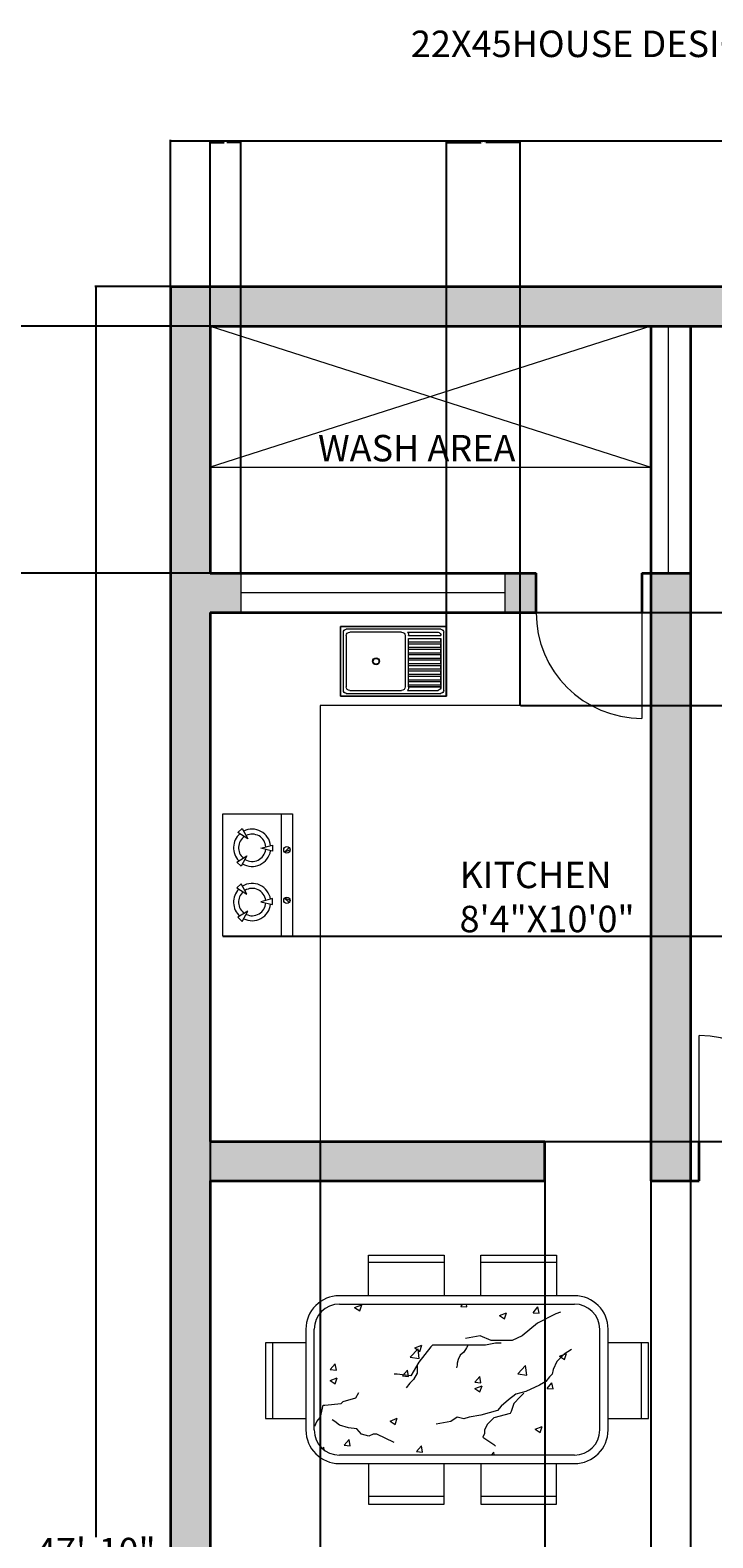
# Model space of a CAD drawing. Units: inches. Extents: x 37 to 706, y -568 to 110.
# Tile 22 of 24: x 362 to 517, y -233 to 110. Entities that reach past the tile are written whole.
import ezdxf

# ---------------------------------------------------------------- set-up
doc = ezdxf.new("R2010")
doc.units = ezdxf.units.IN
doc.header["$MEASUREMENT"] = 0
for name, color, linetype, lineweight in [('A-ANNO-DIMS', 2, 'Continuous', 18), ('A-ANNO-TEXT', 7, 'Continuous', 18), ('A-AREA-IDEN', 7, 'Continuous', 18), ('A-DOOR', 4, 'Continuous', 18), ('A-EQPM', 8, 'Continuous', 18), ('A-FLOR-CASE', 9, 'Continuous', 18), ('A-FLOR-FIXT', 9, 'Continuous', 18), ('A-FLOR-OPEN', 8, 'Continuous', 13), ('A-FURN', 8, 'Continuous', 13), ('A-GLAZ', 4, 'Continuous', 18), ('A-WALL', 7, 'Continuous', 35), ('A-WALL-PATT', 252, 'Continuous', 13)]:
    doc.layers.add(name, color=color, linetype=linetype, lineweight=lineweight)
doc.styles.get("Standard").update_dxf_attribs({"font": 'arial.ttf'})
doc.dimstyles.get("Standard").update_dxf_attribs({"dimtxt": 0.18, "dimasz": 0.18, "dimexe": 0.18, "dimexo": 0.0625, "dimgap": 0.09, "dimtad": 0, "dimtih": 1, "dimtoh": 1, "dimdec": 0, "dimzin": 0, "dimdsep": 46, "dimlunit": 3, "dimtxsty": 'Standard', "dimcen": 0.09, "dimadec": 0, "dimazin": 0, "dimtfac": 1, "dimtdec": 0, "dimtofl": 0, "dimtmove": 0, "dimatfit": 3, "dimfxl": 1, "dimtolj": 1, "dimtzin": 0, "dimarcsym": 0})

# ---------------------------------------------------------------- blocks, each defined once
blk = doc.blocks.new('М12 540х820')
for p, q in [((0, 540), (-820, 540)), ((-820, 540), (-820, 0)), ((-798, 495), (-798, 45)), ((-45, 517), (-775, 517)), ((-775, 468), (-775, 72)), ((-348, 495), (-748, 495)), ((-320, 468), (-320, 72)), ((-302, 495), (-65, 495)), ((-294, 468), (-294, 472)), ((-294, 468), (-45, 468)), ((-45, 470), (-45, 468)), ((-22, 45), (-22, 495)), ((0, 0), (0, 540)), ((-294, 447), (-45, 447)), ((-294, 420), (-294, 447)), ((-294, 420), (-45, 420)), ((-294, 405), (-45, 405)), ((-294, 378), (-294, 405)), ((-294, 378), (-45, 378)), ((-294, 336), (-294, 363)), ((-294, 363), (-45, 363)), ((-45, 420), (-45, 447)), ((-45, 378), (-45, 405)), ((-45, 336), (-45, 363)), ((-294, 336), (-45, 336)), ((-294, 295), (-294, 322)), ((-294, 322), (-45, 322)), ((-294, 295), (-45, 295)), ((-294, 253), (-294, 280)), ((-294, 280), (-45, 280)), ((-294, 253), (-45, 253)), ((-294, 211), (-294, 238)), ((-294, 238), (-45, 238)), ((-45, 295), (-45, 322)), ((-45, 253), (-45, 280)), ((-45, 211), (-45, 238)), ((-294, 211), (-45, 211)), ((-294, 170), (-294, 197)), ((-294, 197), (-45, 197)), ((-294, 170), (-45, 170)), ((-294, 128), (-294, 155)), ((-294, 155), (-45, 155)), ((-294, 128), (-45, 128)), ((-45, 170), (-45, 197)), ((-45, 128), (-45, 155)), ((-820, 0), (0, 0)), ((-775, 22), (-45, 22)), ((-748, 45), (-348, 45)), ((-302, 45), (-65, 45)), ((-294, 114), (-45, 114)), ((-294, 87), (-294, 114)), ((-294, 87), (-45, 87)), ((-294, 72), (-45, 72)), ((-45, 87), (-45, 114)), ((-45, 70), (-45, 72))]:
    blk.add_line(p, q)
at = {"ltscale": 0.06}
for p, q in [((-820, 0), (-820, 540)), ((-820, 540), (0, 540)), ((0, 540), (0, 537)), ((0, 537), (0, 0)), ((-294, 447), (-45, 447)), ((-294, 405), (-294, 447)), ((-294, 363), (-294, 405)), ((-294, 322), (-294, 363)), ((-45, 447), (-45, 420)), ((-45, 420), (-45, 378)), ((-45, 378), (-45, 336)), ((-294, 280), (-294, 322)), ((-294, 238), (-294, 280)), ((-294, 197), (-294, 238)), ((-45, 336), (-45, 295)), ((-45, 295), (-45, 253)), ((-45, 253), (-45, 211)), ((-294, 155), (-294, 197)), ((-294, 114), (-294, 155)), ((-45, 211), (-45, 170)), ((-45, 170), (-45, 128)), ((-45, 128), (-45, 87)), ((0, 0), (-820, 0)), ((-294, 72), (-294, 114)), ((-45, 72), (-294, 72)), ((-45, 87), (-45, 72))]:
    blk.add_line(p, q, dxfattribs=at)
at = {"extrusion": (0, 0, -1)}
for centre, major_axis, start_param, end_param in [((-775, 495), (-15.9, 15.9), -0.785398, 0.785398), ((-775, 495), (-15.9, 15.9), -0.785398, 0.785398), ((-748, 468), (-19.1, -19.1), 0.785398, 2.356194), ((-748, 468), (-19.1, -19.1), 0.785398, 2.356194), ((-348, 468), (-19.1, 19.1), 0.785398, 2.356194), ((-348, 468), (-19.1, 19.1), 0.785398, 2.356194), ((-343, 468), (-35, 35), 1.779263, 2.356194), ((-343, 468), (-35, 35), 1.779263, 2.356192), ((-343, 468), (-35, 35), 2.356192, 2.356194), ((-72, 469), (-19.3, 19.3), 1.0328, 2.38382), ((-72, 469), (-19.3, 19.3), 1.0328, 1.064673), ((-72, 469), (-19.3, 19.3), 1.064673, 2.328569), ((-45, 495), (-15.9, -15.9), 2.356194, 3.926991), ((-45, 495), (-15.9, -15.9), 2.356194, 3.926991), ((-72, 469), (-19.3, 19.3), 2.328569, 2.38382), ((-545, 270), (-19.1, -19.1), 3.926991, 10.210176), ((-545, 270), (-19.1, -19.1), 3.926991, 10.210176), ((-545, 270), (-15.9, -15.9), 3.926991, 10.210176), ((-545, 270), (-15.9, -15.9), 3.926991, 10.210176), ((-775, 45), (-15.9, -15.9), 5.497787, 7.068583), ((-775, 45), (-15.9, -15.9), 5.497787, 7.068583), ((-748, 72), (-19.1, 19.1), 3.926991, 5.497787), ((-748, 72), (-19.1, 19.1), 3.926991, 5.497787), ((-348, 72), (-19.1, -19.1), 3.926991, 5.497787), ((-348, 72), (-19.1, -19.1), 3.926991, 5.497787), ((-343, 72), (-35, -35), 3.926991, 4.503922), ((-343, 72), (-35, -35), 3.926991, 4.503922), ((-72, 71), (-19.3, -19.3), 3.899365, 5.250385), ((-72, 71), (-19.3, -19.3), 5.218512, 5.250385), ((-72, 71), (-19.3, -19.3), 3.954617, 5.218512), ((-72, 71), (-19.3, -19.3), 3.899365, 3.954617), ((-45, 45), (-15.9, 15.9), 2.356194, 3.926991), ((-45, 45), (-15.9, 15.9), 2.356194, 3.926991)]:
    blk.add_ellipse(centre, major_axis=major_axis, ratio=1, start_param=start_param, end_param=end_param, dxfattribs=at)
blk = doc.blocks.new('*D4')
at = {"layer": 'A-ANNO-DIMS', "color": 0, "lineweight": -2, "transparency": 16777216}
for p, q in [((393.96, 51.35), (393.96, 84.59)), ((394.14, 84.41), (523.01, 84.41)), ((672.78, 84.41), (543.91, 84.41)), ((672.96, 51.35), (672.96, 84.59))]:
    blk.add_line(p, q, dxfattribs=at)
at = {"layer": 'A-ANNO-DIMS', "color": 0, "transparency": 16777216}
for points in [[(394.14, 84.44), (394.14, 84.38), (393.96, 84.41)], [(672.78, 84.44), (672.78, 84.38), (672.96, 84.41)]]:
    blk.add_solid(points, dxfattribs=at)
at = {"layer": 'Defpoints', "color": 0, "transparency": 16777216}
for p in [(672.96, 84.41), (393.96, 51.29), (672.96, 51.29)]:
    blk.add_point(p, dxfattribs=at)
at = {"layer": 'A-ANNO-DIMS', "color": 0, "transparency": 16777216, "insert": (533.46, 84.41), "char_height": 6, "attachment_point": 5}
blk.add_mtext('\\A1;23\'-3"', dxfattribs=at)
blk = doc.blocks.new('*D5')
at = {"layer": 'A-ANNO-DIMS', "color": 0, "lineweight": -2, "transparency": 16777216}
for p, q in [((393.9, 51.29), (376.84, 51.29)), ((377.02, 51.11), (377.02, -232.56)), ((377.02, -522.53), (377.02, -238.86)), ((393.9, -522.71), (376.84, -522.71))]:
    blk.add_line(p, q, dxfattribs=at)
at = {"layer": 'A-ANNO-DIMS', "color": 0, "transparency": 16777216}
for points in [[(376.99, 51.11), (377.05, 51.11), (377.02, 51.29)], [(376.99, -522.53), (377.05, -522.53), (377.02, -522.71)]]:
    blk.add_solid(points, dxfattribs=at)
at = {"layer": 'Defpoints', "color": 0, "transparency": 16777216}
for p in [(393.96, 51.29), (377.02, -522.71), (393.96, -522.71)]:
    blk.add_point(p, dxfattribs=at)
at = {"layer": 'A-ANNO-DIMS', "color": 0, "transparency": 16777216, "insert": (377.02, -235.71), "char_height": 6, "attachment_point": 5}
blk.add_mtext('\\A1;47\'-10"', dxfattribs=at)
blk = doc.blocks.new('DINING-SET-6')
for p, q in [((23.4, 47.29), (23.4, 56.48)), ((23.4, 56.48), (40.55, 56.48)), ((40.55, 54.8), (23.4, 54.8)), ((40.55, 56.48), (40.55, 47.29)), ((48.93, 47.29), (48.93, 56.48)), ((48.93, 56.48), (66.08, 56.48)), ((66.08, 54.8), (48.93, 54.8)), ((66.08, 56.48), (66.08, 47.29)), ((70.16, 47.29), (16.81, 47.29)), ((16.81, 45.39), (70.16, 45.39)), ((20.27, 44.63), (21.87, 45.24)), ((20.27, 44.63), (21.41, 43.86)), ((21.41, 43.86), (21.87, 45.24)), ((44.37, 44.86), (44.81, 45.39)), ((44.37, 44.86), (45.74, 44.74)), ((45.74, 44.74), (45.62, 45.39)), ((60.77, 43.43), (61.87, 44.74)), ((62.14, 43.31), (61.87, 44.74)), ((53.13, 42.8), (54.73, 43.41)), ((53.13, 42.8), (54.27, 42.03)), ((54.27, 42.03), (54.73, 43.41)), ((60.77, 43.43), (62.14, 43.31)), ((65.93, 43.13), (61.79, 41.06)), ((66.97, 43.54), (65.93, 43.13)), ((9.18, 39.67), (9.18, 16.81)), ((11.09, 16.81), (11.09, 39.67)), ((46.25, 37.75), (45.42, 37.54)), ((48.74, 38.16), (46.25, 37.75)), ((51.22, 37.13), (48.74, 38.16)), ((58.27, 38.16), (55.99, 37.13)), ((61.79, 41.06), (58.27, 38.16)), ((75.87, 39.67), (75.87, 16.81)), ((77.78, 16.81), (77.78, 39.67)), ((0, 36.58), (0, 19.44)), ((9.18, 36.58), (0, 36.58)), ((1.68, 19.44), (1.68, 36.58)), ((32.89, 33.34), (34.67, 35.2)), ((33.92, 35.42), (35.52, 36.03)), ((33.92, 35.42), (35.05, 34.65)), ((34.92, 33.03), (34.67, 35.2)), ((37.55, 35.68), (34.85, 32.16)), ((35.05, 34.65), (35.52, 36.03)), ((37.96, 36.09), (37.55, 35.68)), ((49.98, 36.09), (37.96, 36.09)), ((45.01, 34.45), (44.18, 33.82)), ((45.63, 35.48), (45.01, 34.45)), ((46.04, 36.1), (45.63, 35.48)), ((52.26, 36.51), (49.98, 36.09)), ((55.99, 37.13), (51.22, 37.13)), ((53.5, 36.51), (52.26, 36.51)), ((69.45, 35.06), (67.8, 34.02)), ((86.96, 36.58), (77.78, 36.58)), ((85.29, 36.58), (85.29, 19.44)), ((86.96, 19.44), (86.96, 36.58)), ((14.74, 30.53), (15.84, 31.85)), ((16.11, 30.41), (15.84, 31.85)), ((32.89, 33.34), (34.92, 33.03)), ((34.85, 32.16), (32.99, 29.06)), ((34.44, 31.54), (34.44, 29.68)), ((43.56, 31.55), (43.35, 30.93)), ((43.77, 32.79), (43.56, 31.96)), ((43.56, 31.96), (43.56, 31.55)), ((44.18, 33.82), (43.77, 32.79)), ((57.29, 29.56), (59.07, 31.41)), ((59.33, 29.24), (59.07, 31.41)), ((66.14, 32.37), (65.31, 30.51)), ((67.8, 34.02), (66.14, 32.37)), ((66.78, 33.59), (68.38, 34.2)), ((66.78, 33.59), (67.91, 32.82)), ((67.91, 32.82), (68.38, 34.2)), ((14.7, 28.05), (16.31, 28.66)), ((14.7, 28.05), (15.84, 27.28)), ((14.74, 30.53), (16.11, 30.41)), ((15.84, 27.28), (16.31, 28.66)), ((29.88, 29.47), (29.26, 29.47)), ((32.99, 29.06), (29.88, 29.47)), ((31.14, 29.1), (32.24, 30.41)), ((31.14, 29.1), (32.51, 28.98)), ((32.78, 27.4), (31.95, 26.37)), ((32.51, 28.98), (32.24, 30.41)), ((33.61, 28.23), (32.78, 27.4)), ((34.44, 29.68), (33.61, 28.23)), ((47.54, 27.66), (48.64, 28.98)), ((47.54, 27.66), (48.91, 27.54)), ((48.91, 27.54), (48.65, 28.98)), ((57.29, 29.56), (59.32, 29.24)), ((63.65, 27.82), (62.2, 26.99)), ((64.48, 28.85), (63.65, 27.82)), ((63.94, 26.23), (65.05, 27.54)), ((65.1, 29.47), (64.48, 28.85)), ((65.31, 26.11), (65.05, 27.54)), ((65.31, 30.51), (65.1, 29.47)), ((17.66, 23.26), (20.56, 24.09)), ((20.56, 24.09), (21.18, 25.33)), ((47.56, 26.21), (49.17, 26.83)), ((47.56, 26.21), (48.7, 25.45)), ((48.7, 25.45), (49.17, 26.83)), ((56.82, 24.92), (55.16, 23.68)), ((57.85, 24.3), (56.4, 22.85)), ((59.09, 25.54), (56.82, 24.92)), ((58.68, 25.13), (57.85, 24.3)), ((62.2, 26.99), (59.09, 25.54)), ((63.94, 26.23), (65.31, 26.11)), ((12.48, 19.74), (13.1, 22.44)), ((13.1, 22.44), (13.51, 22.44)), ((13.51, 22.44), (17.24, 22.85)), ((17.24, 22.85), (17.66, 23.26)), ((52.67, 21.19), (48.94, 20.16)), ((55.57, 20.57), (51.84, 19.54)), ((53.5, 22.23), (52.67, 21.19)), ((55.16, 23.68), (53.5, 22.23)), ((55.78, 20.99), (55.57, 20.57)), ((56.4, 22.85), (55.78, 20.99)), ((0, 19.44), (9.18, 19.44)), ((11.23, 17.68), (11.65, 18.71)), ((11.65, 18.71), (12.48, 19.74)), ((15.79, 18.72), (15.17, 19.13)), ((16.83, 17.89), (15.79, 18.72)), ((18.9, 17.27), (16.83, 17.89)), ((20.77, 17.06), (18.9, 17.27)), ((28.35, 18.84), (29.95, 19.45)), ((28.35, 18.84), (29.49, 18.07)), ((29.49, 18.07), (29.95, 19.45)), ((42.11, 18.71), (38.79, 18.09)), ((43.56, 19.74), (42.11, 18.71)), ((45.01, 19.33), (43.56, 19.74)), ((46.25, 19.74), (45.01, 19.33)), ((48.94, 20.16), (46.25, 19.74)), ((50.39, 18.09), (49.77, 16.85)), ((51.84, 19.54), (50.39, 18.09)), ((61.21, 17.01), (62.81, 17.62)), ((62.35, 16.24), (62.81, 17.62)), ((77.78, 19.44), (86.96, 19.44)), ((17.91, 13.33), (19.02, 14.65)), ((19.28, 13.21), (19.02, 14.65)), ((21.8, 15.82), (20.77, 17.06)), ((23.46, 15.41), (21.8, 15.82)), ((24.5, 15.82), (23.46, 15.41)), ((25.33, 15.82), (24.5, 15.82)), ((29.26, 13.96), (25.33, 15.82)), ((49.77, 16.02), (49.36, 15.19)), ((49.36, 15.19), (51.84, 13.54)), ((49.77, 16.85), (49.77, 16.02)), ((61.21, 17.01), (62.35, 16.24)), ((12.96, 12.57), (13.3, 12.92)), ((13.38, 12.23), (13.3, 12.92)), ((70.16, 11.09), (16.81, 11.09)), ((17.91, 13.33), (19.28, 13.22)), ((34.31, 11.9), (35.42, 13.21)), ((34.31, 11.9), (35.68, 11.78)), ((35.68, 11.78), (35.42, 13.21)), ((51.24, 11.09), (51.82, 11.78)), ((51.94, 11.09), (51.82, 11.78)), ((51.84, 13.54), (52.26, 13.12)), ((16.81, 9.18), (70.16, 9.18)), ((23.4, 9.18), (23.4, 0)), ((40.55, 0), (40.55, 9.18)), ((48.93, 9.18), (48.93, 0)), ((66.08, 0), (66.08, 9.18)), ((40.55, 1.68), (23.4, 1.68)), ((23.4, 0), (40.55, 0)), ((66.08, 1.68), (48.93, 1.68)), ((48.93, 0), (66.08, 0))]:
    blk.add_line(p, q)
for centre, radius, start, end in [((16.81, 39.67), 7.62, 90, 180), ((16.81, 39.67), 5.72, 90, 180), ((70.16, 39.67), 7.62, 0, 90), ((70.16, 39.67), 5.72, 0, 90), ((16.81, 16.81), 7.62, 180, 270), ((16.81, 16.81), 5.72, 180, 270), ((70.16, 16.81), 5.72, 270, 0), ((70.16, 16.81), 7.62, 270, 0)]:
    blk.add_arc(centre, radius, start, end)
blk = doc.blocks.new('COOKTOP-2-BURNER')
for p, q in [((13.28, 27.75), (13.28, 0)), ((3.44, 23.52), (4.41, 24.48)), ((4.41, 24.48), (5.73, 22.12)), ((5.73, 22.12), (3.44, 23.52)), ((8.68, 19.98), (11.28, 20.64)), ((11.28, 20.64), (11.28, 19.27)), ((3.19, 16.84), (5.49, 18.26)), ((5.49, 18.26), (4.19, 15.9)), ((11.28, 19.27), (8.68, 19.98)), ((4.19, 15.9), (3.19, 16.84)), ((4.19, 11.91), (3.19, 10.98)), ((3.19, 10.98), (5.49, 9.56)), ((5.49, 9.56), (4.19, 11.91)), ((11.28, 8.55), (8.68, 7.83)), ((8.68, 7.83), (11.28, 7.18)), ((11.28, 7.18), (11.28, 8.55)), ((5.73, 5.7), (3.44, 4.29)), ((3.44, 4.29), (4.41, 3.33)), ((4.41, 3.33), (5.73, 5.7))]:
    blk.add_line(p, q)
at = {"ltscale": 20}
for p, q in [((14.06, 19.09), (15.09, 20.13)), ((15.3, 19.61), (14.06, 19.09)), ((14.06, 8.66), (15.09, 7.62)), ((15.3, 8.14), (14.06, 8.66))]:
    blk.add_line(p, q, dxfattribs=at)
blk.add_lwpolyline([(0, 0), (0, 27.75), (15.86, 27.75), (15.86, 0)], close=True)
for centre in [(14.57, 19.61), (14.57, 8.14)]:
    blk.add_circle(centre, 0.73, dxfattribs=at)
for centre, radius, start, end in [((6.68, 20.07), 4.23, 6.4005, 116.769), ((6.68, 20.07), 4.23, 131.2225, 224.1627), ((6.68, 20.07), 3.1, 124.5561, 228.8027), ((6.68, 20.07), 3.1, 3.5753, 115.9207), ((6.68, 20.07), 4.23, 238.853, 350.7562), ((6.68, 20.07), 3.1, 237.9778, 353.02), ((6.68, 7.75), 4.23, 135.8373, 228.7775), ((6.68, 7.75), 4.23, 9.2438, 121.147), ((6.68, 7.75), 3.1, 6.98, 122.0222), ((6.68, 7.75), 3.1, 131.1973, 235.4439), ((6.68, 7.75), 4.23, 243.231, 353.5995), ((6.68, 7.75), 3.1, 244.0793, 356.4247)]:
    blk.add_arc(centre, radius, start, end)
blk = doc.blocks.new('WIN-60')
for p, q in [((60, 9), (0, 9)), ((0, 9), (0, 0)), ((60, 0), (60, 9)), ((60, 4.5), (0, 4.5)), ((0, 0), (60, 0))]:
    blk.add_line(p, q)
blk = doc.blocks.new('DOOR-SWING-24')
blk.add_line((0, 0), (0, 24))
blk.add_arc((0, 0), 24, 0, 90)
blk = doc.blocks.new('*D42')
at = {"layer": 'A-ANNO-DIMS', "color": 0, "lineweight": -2, "transparency": 16777216}
for p, q in [((402.9, 42.29), (46.03, 42.29)), ((46.21, 42.11), (46.21, 14.47)), ((46.21, -13.53), (46.21, 14.11)), ((402.9, -13.71), (46.03, -13.71))]:
    blk.add_line(p, q, dxfattribs=at)
at = {"layer": 'A-ANNO-DIMS', "color": 0, "transparency": 16777216}
for points in [[(46.18, 42.11), (46.24, 42.11), (46.21, 42.29)], [(46.18, -13.53), (46.24, -13.53), (46.21, -13.71)]]:
    blk.add_solid(points, dxfattribs=at)
at = {"layer": 'Defpoints', "color": 0, "transparency": 16777216}
for p in [(402.96, 42.29), (46.21, -13.71), (402.96, -13.71)]:
    blk.add_point(p, dxfattribs=at)
at = {"layer": 'A-ANNO-DIMS', "color": 0, "transparency": 16777216, "insert": (46.21, 14.29), "char_height": 0.18, "attachment_point": 5}
blk.add_mtext('\\A1;4\'-8"', dxfattribs=at)
blk = doc.blocks.new('*D53')
at = {"layer": 'A-ANNO-DIMS', "color": 0, "lineweight": -2, "transparency": 16777216}
for p, q in [((511.96, -151.77), (511.96, -567.64)), ((537.96, -151.77), (537.96, -567.64)), ((512.14, -567.46), (524.63, -567.46)), ((537.78, -567.46), (525.29, -567.46))]:
    blk.add_line(p, q, dxfattribs=at)
at = {"layer": 'A-ANNO-DIMS', "color": 0, "transparency": 16777216}
for points in [[(512.14, -567.43), (512.14, -567.49), (511.96, -567.46)], [(537.78, -567.43), (537.78, -567.49), (537.96, -567.46)]]:
    blk.add_solid(points, dxfattribs=at)
at = {"layer": 'Defpoints', "color": 0, "transparency": 16777216}
for p in [(511.96, -151.71), (537.96, -151.71), (537.96, -567.46)]:
    blk.add_point(p, dxfattribs=at)
at = {"layer": 'A-ANNO-DIMS', "color": 0, "transparency": 16777216, "insert": (524.96, -567.46), "char_height": 0.18, "attachment_point": 5}
blk.add_mtext('\\A1;2\'-2"', dxfattribs=at)
blk = doc.blocks.new('*D55')
at = {"layer": 'A-ANNO-DIMS', "color": 0, "lineweight": -2, "transparency": 16777216}
for p, q in [((402.96, -13.65), (402.96, 84.22)), ((403.14, 84.04), (406.13, 84.04)), ((409.78, 84.04), (406.79, 84.04)), ((409.96, -13.65), (409.96, 84.22))]:
    blk.add_line(p, q, dxfattribs=at)
at = {"layer": 'A-ANNO-DIMS', "color": 0, "transparency": 16777216}
for points in [[(403.14, 84.07), (403.14, 84.01), (402.96, 84.04)], [(409.78, 84.07), (409.78, 84.01), (409.96, 84.04)]]:
    blk.add_solid(points, dxfattribs=at)
at = {"layer": 'Defpoints', "color": 0, "transparency": 16777216}
for p in [(409.96, 84.04), (402.96, -13.71), (409.96, -13.71)]:
    blk.add_point(p, dxfattribs=at)
at = {"layer": 'A-ANNO-DIMS', "color": 0, "transparency": 16777216, "insert": (406.46, 84.04), "char_height": 0.18, "attachment_point": 5}
blk.add_mtext('\\A1;0\'-7"', dxfattribs=at)
blk = doc.blocks.new('*D56')
at = {"layer": 'A-ANNO-DIMS', "color": 0, "lineweight": -2, "transparency": 16777216}
for p, q in [((402.96, -142.77), (402.96, -567.64)), ((427.97, -142.77), (427.97, -567.64)), ((403.14, -567.46), (415.13, -567.46)), ((427.79, -567.46), (415.79, -567.46))]:
    blk.add_line(p, q, dxfattribs=at)
at = {"layer": 'A-ANNO-DIMS', "color": 0, "transparency": 16777216}
for points in [[(403.14, -567.43), (403.14, -567.49), (402.96, -567.46)], [(427.79, -567.43), (427.79, -567.49), (427.97, -567.46)]]:
    blk.add_solid(points, dxfattribs=at)
at = {"layer": 'Defpoints', "color": 0, "transparency": 16777216}
for p in [(402.96, -142.71), (427.97, -142.71), (427.97, -567.46)]:
    blk.add_point(p, dxfattribs=at)
at = {"layer": 'A-ANNO-DIMS', "color": 0, "transparency": 16777216, "insert": (415.46, -567.46), "char_height": 0.18, "attachment_point": 5}
blk.add_mtext('\\A1;2\'-1"', dxfattribs=at)
blk = doc.blocks.new('*D57')
at = {"layer": 'A-ANNO-DIMS', "color": 0, "lineweight": -2, "transparency": 16777216}
for p, q in [((473.38, -22.71), (705.89, -22.71)), ((705.71, -22.89), (705.71, -33.06)), ((705.71, -43.59), (705.71, -33.42)), ((473.38, -43.77), (705.89, -43.77))]:
    blk.add_line(p, q, dxfattribs=at)
at = {"layer": 'A-ANNO-DIMS', "color": 0, "transparency": 16777216}
for points in [[(705.68, -22.89), (705.74, -22.89), (705.71, -22.71)], [(705.68, -43.59), (705.74, -43.59), (705.71, -43.77)]]:
    blk.add_solid(points, dxfattribs=at)
at = {"layer": 'Defpoints', "color": 0, "transparency": 16777216}
for p in [(473.32, -22.71), (473.32, -43.77), (705.71, -43.77)]:
    blk.add_point(p, dxfattribs=at)
at = {"layer": 'A-ANNO-DIMS', "color": 0, "transparency": 16777216, "insert": (705.71, -33.24), "char_height": 0.18, "attachment_point": 5}
blk.add_mtext('\\A1;1\'-9"', dxfattribs=at)
blk = doc.blocks.new('*D58')
at = {"layer": 'A-ANNO-DIMS', "color": 0, "lineweight": -2, "transparency": 16777216}
for p, q in [((405.88, -96.15), (705.89, -96.15)), ((705.71, -96.33), (705.71, -119.25)), ((705.71, -142.53), (705.71, -119.61)), ((403.02, -142.71), (705.89, -142.71))]:
    blk.add_line(p, q, dxfattribs=at)
at = {"layer": 'A-ANNO-DIMS', "color": 0, "transparency": 16777216}
for points in [[(705.68, -96.33), (705.74, -96.33), (705.71, -96.15)], [(705.68, -142.53), (705.74, -142.53), (705.71, -142.71)]]:
    blk.add_solid(points, dxfattribs=at)
at = {"layer": 'Defpoints', "color": 0, "transparency": 16777216}
for p in [(405.82, -96.15), (705.71, -96.15), (402.96, -142.71)]:
    blk.add_point(p, dxfattribs=at)
at = {"layer": 'A-ANNO-DIMS', "color": 0, "transparency": 16777216, "insert": (705.71, -119.43), "char_height": 0.18, "attachment_point": 5}
blk.add_mtext('\\A1;3\'-10 1/2"', dxfattribs=at)
blk = doc.blocks.new('*D59')
at = {"layer": 'A-ANNO-DIMS', "color": 0, "lineweight": -2, "transparency": 16777216}
for p, q in [((456.64, -41.62), (456.64, 84.22)), ((456.82, 84.04), (464.45, 84.04)), ((473.14, 84.04), (465.51, 84.04)), ((473.32, -43.71), (473.32, 84.22))]:
    blk.add_line(p, q, dxfattribs=at)
at = {"layer": 'A-ANNO-DIMS', "color": 0, "transparency": 16777216}
for points in [[(456.82, 84.07), (456.82, 84.01), (456.64, 84.04)], [(473.14, 84.07), (473.14, 84.01), (473.32, 84.04)]]:
    blk.add_solid(points, dxfattribs=at)
at = {"layer": 'Defpoints', "color": 0, "transparency": 16777216}
for p in [(456.64, 84.04), (456.64, -41.68), (473.32, -43.77)]:
    blk.add_point(p, dxfattribs=at)
at = {"layer": 'A-ANNO-DIMS', "color": 0, "transparency": 16777216, "insert": (464.98, 84.04), "char_height": 0.18, "attachment_point": 5}
blk.add_mtext('\\A1;1\'-4 1/2"', dxfattribs=at)
blk = doc.blocks.new('*D63')
at = {"layer": 'A-ANNO-DIMS', "color": 0, "lineweight": -2, "transparency": 16777216}
for p, q in [((478.96, -142.77), (478.96, -567.64)), ((502.96, -151.77), (502.96, -567.64)), ((479.14, -567.46), (490.63, -567.46)), ((502.78, -567.46), (491.29, -567.46))]:
    blk.add_line(p, q, dxfattribs=at)
at = {"layer": 'A-ANNO-DIMS', "color": 0, "transparency": 16777216}
for points in [[(479.14, -567.43), (479.14, -567.49), (478.96, -567.46)], [(502.78, -567.43), (502.78, -567.49), (502.96, -567.46)]]:
    blk.add_solid(points, dxfattribs=at)
at = {"layer": 'Defpoints', "color": 0, "transparency": 16777216}
for p in [(478.96, -142.71), (502.96, -151.71), (502.96, -567.46)]:
    blk.add_point(p, dxfattribs=at)
at = {"layer": 'A-ANNO-DIMS', "color": 0, "transparency": 16777216, "insert": (490.96, -567.46), "char_height": 0.18, "attachment_point": 5}
blk.add_mtext('\\A1;2\'-0"', dxfattribs=at)

msp = doc.modelspace()

# ---------------------------------------------------------------- hatches: boundary and pattern name
at = {"layer": 'A-WALL-PATT'}
h = msp.add_hatch(color=256, dxfattribs=at)
h.dxf.hatch_style = 1
h.paths.add_polyline_path([(220.96, -351.71), (211.96, -351.71), (211.96, -513.71), (254.96, -513.71), (254.96, -504.71), (220.96, -504.71)], flags=17)
h.paths.add_polyline_path([(220.96, -294.71), (211.96, -294.71), (211.96, -303.71), (220.96, -303.71)], flags=17)
h.paths.add_polyline_path([(175.96, -294.71), (155.87, -294.71), (155.87, -303.71), (155.96, -303.71), (175.96, -303.71)], flags=17)
h.paths.add_polyline_path([(220.96, -16.71), (211.96, -16.71), (211.96, -142.71), (220.96, -142.71)], flags=17)
h.paths.add_polyline_path([(357.96, 51.29), (78.96, 51.29), (78.96, -513.71), (87.96, -513.71), (87.96, -303.71), (95.87, -303.71), (95.87, -294.71), (87.96, -294.71), (87.96, -142.71), (187.96, -142.71), (187.96, -133.71), (87.96, -133.71), (87.96, -25.71), (106.96, -25.71), (106.96, -16.71), (87.96, -16.71), (87.96, 42.29), (348.96, 42.29), (348.96, 17.13), (348.96, -133.71), (246.96, -133.71), (246.96, -142.71), (348.96, -142.71), (348.96, -294.71), (251.96, -294.71), (251.96, -303.71), (348.96, -303.71), (348.96, -351.71), (260.96, -351.71), (260.96, -329.71), (251.96, -329.71), (251.96, -360.71), (327.45, -360.71), (348.96, -360.71), (348.96, -504.71), (314.96, -504.71), (314.96, -513.71), (357.96, -513.71)])
h.paths.add_polyline_path([(416.96, -303.71), (402.96, -303.71), (402.96, -151.71), (478.96, -151.71), (478.96, -142.71), (402.96, -142.71), (402.96, -22.71), (409.96, -22.71), (409.96, -13.71), (402.96, -13.71), (402.96, 42.29), (663.96, 42.29), (663.96, -303.71), (566.96, -303.71), (566.96, -312.71), (663.96, -312.71), (663.96, -360.71), (575.96, -360.71), (575.96, -338.71), (566.96, -338.71), (566.96, -360.71), (566.96, -369.71), (642.45, -369.71), (663.96, -369.71), (663.96, -513.71), (629.96, -513.71), (629.96, -522.71), (672.96, -522.71), (672.96, 51.29), (393.96, 51.29), (393.96, -522.71), (402.96, -522.71), (402.96, -312.71), (416.96, -312.71)])
h.paths.add_polyline_path([(490.96, -303.71), (476.96, -303.71), (476.96, -312.71), (490.96, -312.71)], flags=17)
h.paths.add_polyline_path([(535.96, -303.71), (526.96, -303.71), (526.96, -312.71), (535.96, -312.71)], flags=17)
h.paths.add_polyline_path([(535.96, -369.71), (526.96, -369.71), (526.96, -522.71), (569.96, -522.71), (569.96, -513.71), (535.96, -513.71)], flags=17)
h.paths.add_polyline_path([(511.96, -13.71), (502.96, -13.71), (502.96, -151.71), (511.96, -151.71)], flags=17)
h.paths.add_polyline_path([(651.54, -142.71), (651.54, -120.18), (642.54, -120.18), (642.54, -142.71), (550.54, -142.71), (550.54, -120.71), (541.54, -120.71), (541.54, -142.71), (537.96, -142.71), (537.96, -151.71), (651.54, -151.71)], flags=17)
h.paths.add_polyline_path([(651.54, -85.71), (541.54, -85.71), (541.54, -94.71), (651.54, -94.71)], flags=17)
h.paths.add_polyline_path([(476.96, -13.71), (469.96, -13.71), (469.96, -22.71), (476.96, -22.71)], flags=17)
h.paths.add_polyline_path([(185.96, -16.71), (166.96, -16.71), (166.96, -25.71), (185.96, -25.71)], flags=17)
h.paths.add_polyline_path([(168.91, -414.72), (214.62, -414.72), (214.62, -392.33), (168.91, -392.33)], flags=25)

# ---------------------------------------------------------------- linework, layer by layer
at = {"layer": 'A-FLOR-CASE'}
for p, q in [((473.32, -22.71), (473.32, -43.77)), ((473.32, -43.77), (427.97, -43.77)), ((427.97, -43.77), (427.97, -142.71))]:
    msp.add_line(p, q, dxfattribs=at)
at = {"layer": 'A-FLOR-OPEN'}
for p, q in [((402.96, 42.29), (502.96, 10.29)), ((502.96, 42.29), (402.96, 10.29)), ((402.96, 10.29), (502.96, 10.29))]:
    msp.add_line(p, q, dxfattribs=at)
at = {"layer": 'A-GLAZ'}
msp.add_line((506.96, -13.71), (506.96, 42.29), dxfattribs=at)
at = {"layer": 'A-WALL'}
for p, q in [((393.96, 51.29), (393.96, -522.71)), ((393.96, 51.29), (672.96, 51.29)), ((402.96, 42.29), (402.96, -13.71)), ((402.96, 42.29), (663.96, 42.29)), ((502.96, 42.29), (502.96, -151.71)), ((511.96, 42.29), (511.96, -151.71)), ((402.96, -13.71), (476.96, -13.71)), ((476.96, -22.71), (476.96, -13.71)), ((500.96, -13.71), (500.96, -22.71)), ((500.96, -13.71), (502.96, -13.71)), ((501.96, -13.71), (511.96, -13.71)), ((402.96, -22.71), (476.96, -22.71)), ((402.96, -22.71), (402.96, -142.71)), ((402.96, -142.71), (478.96, -142.71)), ((478.96, -151.71), (478.96, -142.71)), ((513.96, -151.71), (513.96, -142.71)), ((402.96, -151.71), (478.96, -151.71)), ((402.96, -151.71), (402.96, -303.71)), ((502.96, -151.71), (513.96, -151.71))]:
    msp.add_line(p, q, dxfattribs=at)

# ---------------------------------------------------------------- block references
at = {"layer": 'A-DOOR', "rotation": 180}
msp.add_blockref('DOOR-SWING-24', (500.96, -22.71), dxfattribs=at)
at = {"layer": 'A-DOOR'}
msp.add_blockref('DOOR-SWING-24', (513.96, -142.71), dxfattribs=at)
at = {"layer": 'A-EQPM'}
msp.add_blockref('COOKTOP-2-BURNER', (405.82, -96.15), dxfattribs=at)
at = {"layer": 'A-FLOR-FIXT', "xscale": 0.0293785137493104, "yscale": 0.0293785137493104, "zscale": 0.0293785137493104}
msp.add_blockref('М12 540х820', (456.64, -41.68), dxfattribs=at)
at = {"layer": 'A-FURN'}
msp.add_blockref('DINING-SET-6', (415.5, -225.03), dxfattribs=at)
at = {"layer": 'A-GLAZ'}
msp.add_blockref('WIN-60', (409.96, -22.71), dxfattribs=at)

# ---------------------------------------------------------------- texts
at = {"layer": 'A-ANNO-TEXT', "insert": (448.53, 109.4), "char_height": 6, "attachment_point": 1}
msp.add_mtext_dynamic_manual_height_columns('22X45HOUSE DESIGN WITH CAR PARKING', width=232.4288, gutter_width=1, heights=[0], dxfattribs=at)
at = {"layer": 'A-AREA-IDEN', "char_height": 6, "attachment_point": 1}
for s, insert in [('WASH AREA', (427.45, 17.63)), ('KITCHEN\\P8\'4"X10\'0"', (459.57, -79.24))]:
    msp.add_mtext(s, dxfattribs=dict(at, insert=insert))

# ---------------------------------------------------------------- dimensions: what is measured, and where the dimension line sits
at = {"layer": 'A-ANNO-DIMS'}
for base, p1, p2, override, picture, middle in [((672.96, 84.41), (393.96, 51.29), (672.96, 51.29), {"dimtxt": 6, "dimclrd": 0, "dimclre": 0, "dimclrt": 0}, '*D4', (533.46, 84.41)), ((409.96, 84.04), (402.96, -13.71), (409.96, -13.71), {"dimdec": 1, "dimlfac": 1, "dimrnd": 0, "dimzin": 1, "dimdsep": 46, "dimlunit": 4, "dimfrac": 2}, '*D55', (406.46, 84.04)), ((456.64, 84.04), (473.32, -43.77), (456.64, -41.68), {"dimdec": 1, "dimlfac": 1, "dimrnd": 0, "dimzin": 1, "dimdsep": 46, "dimlunit": 4, "dimfrac": 2}, '*D59', (464.98, 84.04)), ((427.97, -567.46), (402.96, -142.71), (427.97, -142.71), {"dimdec": 1, "dimlfac": 1, "dimrnd": 0, "dimzin": 1, "dimdsep": 46, "dimlunit": 4, "dimfrac": 2}, '*D56', (415.46, -567.46)), ((502.96, -567.46), (478.96, -142.71), (502.96, -151.71), {"dimdec": 1, "dimlfac": 1, "dimrnd": 0, "dimzin": 1, "dimdsep": 46, "dimlunit": 4, "dimfrac": 2}, '*D63', (490.96, -567.46)), ((537.96, -567.46), (511.96, -151.71), (537.96, -151.71), {"dimdec": 1, "dimlfac": 1, "dimrnd": 0, "dimzin": 1, "dimdsep": 46, "dimlunit": 4, "dimfrac": 2}, '*D53', (524.96, -567.46))]:
    dim = msp.add_linear_dim(base=base, p1=p1, p2=p2, dimstyle='Standard', override=override, dxfattribs=at)
    dim.commit()
    dim.dimension.update_dxf_attribs({"geometry": picture, "text_midpoint": middle})
for base, p1, p2, override, picture, middle in [((377.02, -522.71), (393.96, 51.29), (393.96, -522.71), {"dimtxt": 6, "dimclrd": 0, "dimclre": 0, "dimclrt": 0}, '*D5', (377.02, -235.71)), ((46.21, -13.71), (402.96, 42.29), (402.96, -13.71), {"dimdec": 1, "dimlfac": 1, "dimrnd": 0, "dimzin": 1, "dimdsep": 46, "dimlunit": 4, "dimfrac": 2}, '*D42', (46.21, 14.29)), ((705.71, -43.77), (473.32, -22.71), (473.32, -43.77), {"dimdec": 1, "dimlfac": 1, "dimrnd": 0, "dimzin": 1, "dimdsep": 46, "dimlunit": 4, "dimfrac": 2}, '*D57', (705.71, -33.24)), ((705.71, -96.15), (402.96, -142.71), (405.82, -96.15), {"dimdec": 1, "dimlfac": 1, "dimrnd": 0, "dimzin": 1, "dimdsep": 46, "dimlunit": 4, "dimfrac": 2}, '*D58', (705.71, -119.43))]:
    dim = msp.add_linear_dim(base=base, p1=p1, p2=p2, angle=90, dimstyle='Standard', override=override, dxfattribs=at)
    dim.commit()
    dim.dimension.update_dxf_attribs({"geometry": picture, "text_midpoint": middle})

doc.saveas('drawing.dxf')
